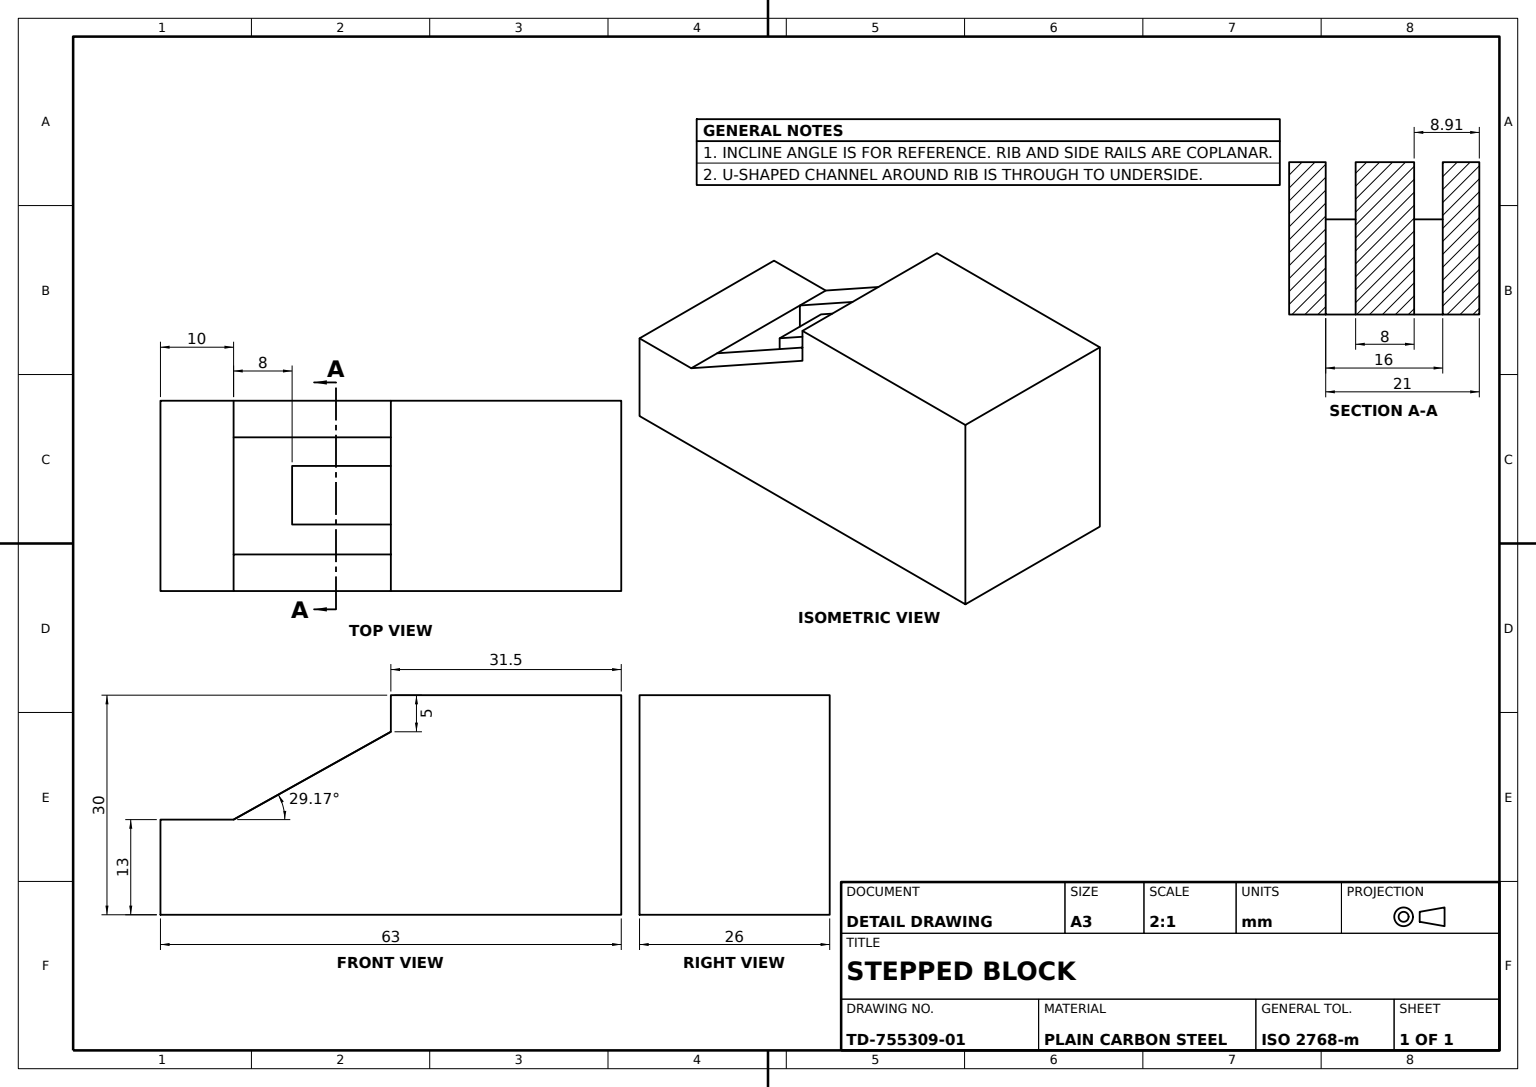
SolidWorks part; units mm, degrees
material "Plain Carbon Steel"
ref_plane "Front Plane" through (0, 0, 0) normal (0, 0, 1) x (1, 0, 0)
ref_plane "Top Plane" through (0, 0, 0) normal (0, 1, 0) x (1, 0, 0)
ref_plane "Right Plane" through (0, 0, 0) normal (1, 0, 0) x (0, 0, -1)
sketch "Base Block Profile" plane through (0, 0, 0) normal (1, 0, 0) x (0, 0, -1)
  line L1 (-31.5, 15) -> (31.5, 15)
  line L2 (-31.5, 15) -> (-31.5, -15)
  line L3 (-31.5, -15) -> (31.5, -15)
  line L4 (31.5, 15) -> (31.5, -15)
  line L5 (-31.5, 15) -> (31.5, -15) construction
  line L6 (-31.5, -15) -> (31.5, 15) construction
  point P0 (0, 0)
  dimension "D1" = 30
  dimension "D2" = 63
extrude "Base Block" add sketch "Base Block Profile" along normal blind 26
sketch "Stepped Slope Profile" plane through (26, 0, 0) normal (1, 0, 0) x (0, 0, -1)
  line L0 (-31.5, -15) -> (-31.5, -2)
  line L1 (-31.5, 15) -> (-31.5, -15) construction
  line L2 (-31.5, -2) -> (-21.5, -2)
  line L3 (-21.5, -2) -> (-21.5, -5)
  line L4 (-21.5, -5) -> (21.5, -5)
  line L5 (21.5, -5) -> (21.5, 5)
  line L6 (21.5, 5) -> (0, 5)
  line L7 (0, 5) -> (0, 15)
  line L8 (31.5, 15) -> (-31.5, 15) construction
  line L9 (-21.5, -2) -> (0, 10)
  line L10 (-31.5, -2) -> (-31.5, 15)
  line L11 (-31.5, 15) -> (0, 15)
  line L12 (31.5, -15) -> (31.5, 15) construction
  line M2 (31.5, 15) -> (-31.5, 15)
  line M3 (-31.5, 15) -> (-31.5, -15)
  dimension "D1" = 10
  dimension "D2" = 13
  dimension "D3" = 10
  dimension "D4" = 10
  dimension "D5" = 10
  dimension "D6" = 31.5
  dimension "D7" = 5
extrude "Stepped Slope Cut" cut sketch "Stepped Slope Profile" against normal blind 26 contours L2 L9 L7 M2 M3
sketch "Inclined Channel Profile" plane through (0, 15, 0) normal (0, 1, 0) x (1, 0, 0)
  line L0 (0, 0) -> (26, 0) construction
  line L1 (5, 0) -> (8.9084, 0)
  line L2 (5, 0) -> (5, -21.5)
  line L3 (5, -21.5) -> (21, -21.5)
  line L4 (21, 0) -> (21, -21.5)
  line L5 (0, -21.5) -> (26, -21.5) construction
  line L6 (16.9084, 0) -> (21, 0)
  line L7 (8.9084, 10.5) -> (16.9084, 10.5)
  line L8 (8.9084, 10.5) -> (8.9084, -13.5)
  line L9 (8.9084, -13.5) -> (16.9084, -13.5)
  line L10 (16.9084, 10.5) -> (16.9084, -13.5)
  line L11 (0, 31.5) -> (0, 0) construction
  line M10 (0, 0) -> (26, 0)
  dimension "D1" = 16
  dimension "D2" = 5
  dimension "D3" = 21
  dimension "D4" = 24
  dimension "D5" = 8
  dimension "D6" = 8.9084
extrude "Inclined Channel Cut" cut sketch "Inclined Channel Profile" against normal blind 44 contours L10 L9 L8 L2 L3 L4 M10
sketch "Notch Reference Sketch" plane through (26, 0, 0) normal (1, 0, 0) x (0, 0, -1)
  line L0 (-21.5, -2) -> (-21.5, -5)
  line L1 (0, 15) -> (31.5, 15)
  line L2 (0, 15) -> (0, 5)
  line L3 (0, 5) -> (31.5, 5)
  line L4 (31.5, 15) -> (31.5, 5)
  line L5 (-21.5, -5) -> (22.9681, -5)
  line L6 (22.9681, -5) -> (22.9681, 5)
  line L7 (-21.5, -5) -> (-21.5, -2)
  line L8 (-21.5, -2) -> (0, 10)
  line L9 (0, 10) -> (0, 5)
  dimension "D1" = 10
  dimension "D2" = 3
  dimension "D3" = 31.5
  dimension "D4" = 44.4681
sketch "Rib Reference Sketch" plane through (0, 15, 0) normal (0, 1, 0) x (1, 0, 0)
  line L0 (16.9084, 0) -> (16.9084, 11.5362)
  line L1 (16.9084, 11.5362) -> (8.9084, 11.5362)
  line L2 (8.9084, 11.5362) -> (8.9084, 0)
  line L3 (0, 0) -> (26, 0) construction
  line L4 (8.9084, 0) -> (16.9084, 0) construction
  line L5 (0, 31.5) -> (0, 0) construction
  dimension "D1" = 8.9084
  dimension "D2" = 19.9638
sketch "Centre Rib Profile" plane through (0, -15, 0) normal (0, -1, 0) x (1, 0, 0)
  line L1 (8.9084, 13.5) -> (16.9084, 13.5)
  line L2 (8.9084, 13.5) -> (8.9084, -11.5362)
  line L3 (8.9084, -11.5362) -> (16.9084, -11.5362)
  line L4 (16.9084, 13.5) -> (16.9084, -11.5362)
extrude "Centre Rib" add sketch "Centre Rib Profile" against normal blind 30
sketch "Notch Profile" plane through (16.9084, 0, 0) normal (1, 0, 0) x (0, 0, -1)
  line L0 (0, 10) -> (-13.5, 2.4651)
  line L1 (-21.5, -2) -> (0, 10) construction
  line L2 (-13.5, -15) -> (-13.5, 15) construction
  line L3 (-13.5, 2.4651) -> (-13.5, 15)
  line L4 (-13.5, 15) -> (0, 15)
  line L5 (0, 15) -> (0, 10)
extrude "Top Notch Cut" cut sketch "Notch Profile" against normal blind 30
